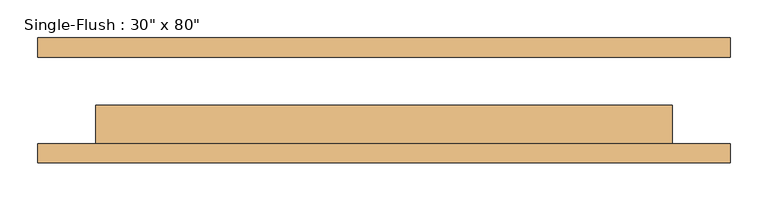
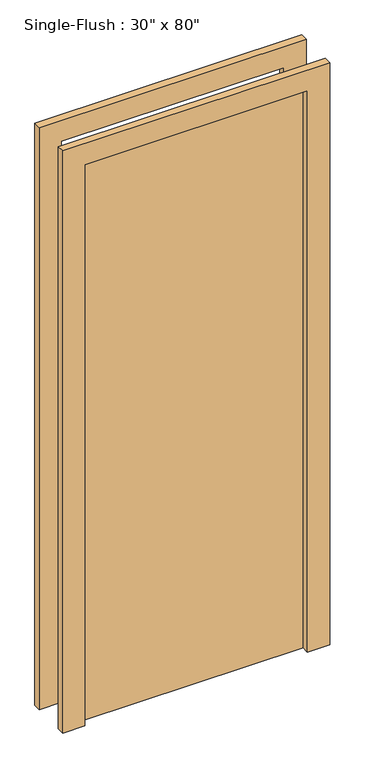
"""IFC4 building model written with IfcOpenShell, lengths in millimetres: door geometry."""

from ifc_helpers import new_model, si_unit, frame, origin, origin_with_axes, place, context, project, spatial, polyline, outline, extrude, source, transform, mapped, element, save


def door_f2b275c1(model_context):
    return source(origin(), model_context, "Body", "SweptSolid", [
        extrude(outline(polyline([(2108.2, -457.2), (0.0, -457.2), (0.0, -381.0), (2032.0, -381.0), (2032.0, 381.0), (0.0, 381.0), (0.0, 457.2), (2108.2, 457.2), (2108.2, -457.2)])), frame((0.0, -82.55, 0.0), z_axis=(0.0, 1.0, 0.0), x_axis=(0.0, 0.0, 1.0)), (0.0, 0.0, 1.0), 25.4),
        extrude(outline(polyline([(2108.2, 457.2), (2108.2, -457.2), (0.0, -457.2), (0.0, -381.0), (2032.0, -381.0), (2032.0, 381.0), (0.0, 381.0), (0.0, 457.2), (2108.2, 457.2)])), frame((0.0, 57.15, 0.0), z_axis=(0.0, 1.0, 0.0), x_axis=(0.0, 0.0, 1.0)), (0.0, 0.0, 1.0), 25.4),
        extrude(outline(polyline([(381.0, -6.35), (381.0, -57.15), (-381.0, -57.15), (-381.0, -6.35), (381.0, -6.35)])), origin_with_axes(), (0.0, 0.0, 1.0), 2032.0),
    ])


if __name__ == "__main__":
    model = new_model("IFC4")
    model_context = context("Model", 3, world=origin())
    ifc_project = project(units=[si_unit("LENGTHUNIT", "METRE", prefix="MILLI")], contexts=[model_context])
    site = spatial("IfcSite", under=ifc_project)
    building = spatial("IfcBuilding", under=site)
    placement = place(None, origin())
    door_shape = door_f2b275c1(model_context)
    element("IfcDoor", 1, ObjectType="Single-Flush : 30\" x 80\"", at=placement, inside=building, context=model_context, shape_type="MappedRepresentation", body=[
        mapped(door_shape, transform((0.0, 0.0, 0.0), x_axis=(1.0, 0.0, 0.0), y_axis=(0.0, 1.0, 0.0), z_axis=(0.0, 0.0, 1.0))),
    ])
    save(model, "model.ifc")

# Revit data of these elements
# Type "Single-Flush : 30\" x 80\""
#   Type Mark = "5"
#   Construction Type Id = "MDOOR"
#   Assembly Code = "C1020"
#   Analytic Construction = "Metal"
#   Thickness = 0' - 2"
#   Heat Transfer Coefficient (U) = 0.651978 BTU/(h·ft²·°F)
#   Height = 6' - 8"
#   Trim Projection Ext = 0' - 1"
#   Trim Projection Int = 0' - 1"
#   Trim Width = 0' - 3"
#   Width = 2' - 6"
#   Define Thermal Properties by = 1
#   Define Thermal Properties by = 1
#   Door Material = Door - Panel
#   Frame Material = Door - Frame
#   Visual Light Transmittance = 0
#   Solar Heat Gain Coefficient = 0
#   Function = (empty or 0)
#   Wall Closure = (empty or 0)
# Element 1 (IfcDoor, "Single-Flush : 30\" x 80\"")
#   Materials on its faces: "Door - Frame", "Door - Panel"
# Materials
#   "Door - Panel": class "Wood", colour RGB 210 159 95, transparency 0, Cost = 0
#   "Door - Frame": colour RGB 118 70 51, transparency 0, Cost = 0
